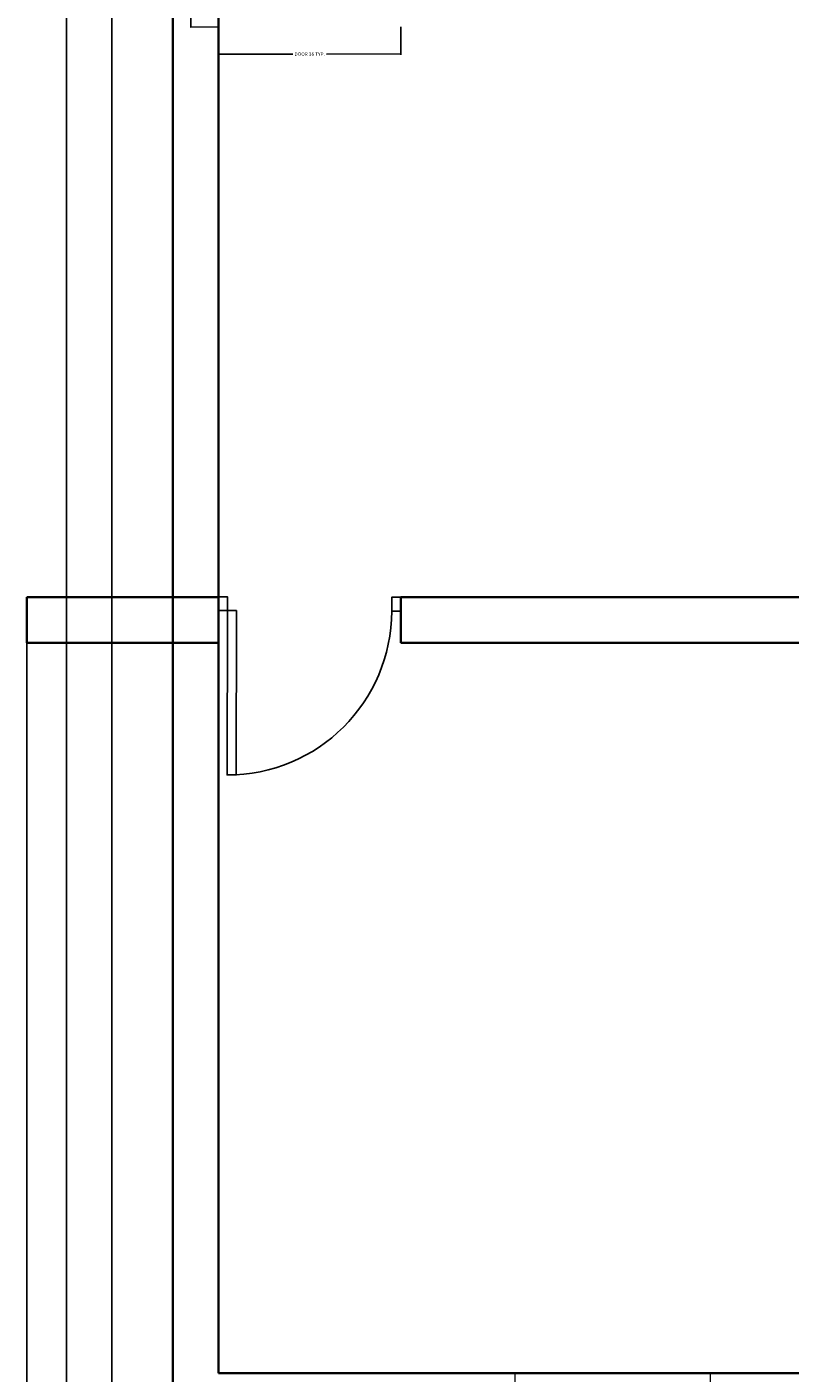
# Model space of a CAD drawing. Units: inches. Extents: x 867 to 1667, y -234 to 788.
# Tile 24 of 42: x 1366 to 1517, y -8 to 258. Entities that reach past the tile are written whole.
import ezdxf

# ---------------------------------------------------------------- set-up
doc = ezdxf.new("R2010")
doc.units = ezdxf.units.IN
doc.header["$MEASUREMENT"] = 0
for name, color, linetype, lineweight in [('A-ANNO-DIMS', 2, 'Continuous', 18), ('A-Door', 150, 'Continuous', 25), ('A-Glaz', 92, 'Continuous', 18), ('A-Wall', 7, 'Continuous', 35)]:
    doc.layers.add(name, color=color, linetype=linetype, lineweight=lineweight)
doc.layers.add('NET 01', color=8, linetype='Continuous')
doc.styles.get("Standard").update_dxf_attribs({"font": 'arial.ttf'})
doc.dimstyles.get("Standard").update_dxf_attribs({"dimtxt": 0.6875, "dimasz": 0.18, "dimexe": 0.18, "dimexo": 0.0625, "dimgap": 0.09, "dimtad": 0, "dimdec": 4, "dimzin": 0, "dimdsep": 46, "dimlunit": 4, "dimtxsty": 'Standard', "dimcen": 0.09, "dimadec": 0, "dimazin": 0, "dimtfac": 1, "dimtdec": 4, "dimtofl": 0, "dimtmove": 0, "dimatfit": 3, "dimfxl": 1, "dimtolj": 1, "dimtzin": 0, "dimarcsym": 0})

# ---------------------------------------------------------------- blocks, each defined once
blk = doc.blocks.new('A$C292B336C')
at = {"layer": 'A-Door'}
for points in [[(-0.05, 0), (-0.05, 0.9), (0, 0.9), (0, 0)], [(-0.95, 0), (-0.95, -0.075), (-0.9, -0.075), (-0.9, 0)], [(0, 0), (0, -0.075), (0.05, -0.075), (0.05, 0)]]:
    blk.add_lwpolyline(points, close=True, dxfattribs=at)
at = {"layer": 'NET 01'}
blk.add_arc((0, 0), 0.9, 90, 180, dxfattribs=at)
blk = doc.blocks.new('WIN-38_58IN')
for p, q in [((0, 9), (0, 0)), ((38.58, 0), (38.58, 9)), ((0, 6), (38.58, 6)), ((0, 2.92), (38.58, 2.92)), ((0, 0), (38.58, 0))]:
    blk.add_line(p, q)
blk = doc.blocks.new('*D5')
at = {"layer": 'A-ANNO-DIMS', "color": 0, "lineweight": -2, "transparency": 16777216}
for p, q in [((1403.89, 257.55), (1403.9, 252.04)), ((1439.9, 257.64), (1439.91, 252.12)), ((1404.08, 252.22), (1418.58, 252.25)), ((1439.73, 252.3), (1425.22, 252.26))]:
    blk.add_line(p, q, dxfattribs=at)
at = {"layer": 'A-ANNO-DIMS', "color": 0, "transparency": 16777216}
for points in [[(1404.08, 252.25), (1404.08, 252.19), (1403.9, 252.22)], [(1439.73, 252.33), (1439.73, 252.27), (1439.91, 252.3)]]:
    blk.add_solid(points, dxfattribs=at)
at = {"layer": 'Defpoints', "color": 0, "transparency": 16777216}
for p in [(1403.89, 257.62), (1439.9, 257.7), (1403.9, 252.22)]:
    blk.add_point(p, dxfattribs=at)
at = {"layer": 'A-ANNO-DIMS', "color": 0, "transparency": 16777216, "insert": (1421.9, 252.26), "char_height": 0.6875, "attachment_point": 5, "rotation": 0.1281}
blk.add_mtext('\\A1;DOOR 36 TYP.', dxfattribs=at)
blk = doc.blocks.new('*D6')
at = {"layer": 'A-ANNO-DIMS', "color": 0, "lineweight": -2, "transparency": 16777216}
for p, q in [((1403.75, 292.73), (1398.23, 292.72)), ((1398.41, 292.54), (1398.44, 276.92)), ((1398.48, 257.78), (1398.45, 273.4)), ((1403.82, 257.62), (1398.3, 257.6))]:
    blk.add_line(p, q, dxfattribs=at)
at = {"layer": 'A-ANNO-DIMS', "color": 0, "transparency": 16777216}
for points in [[(1398.44, 292.54), (1398.38, 292.54), (1398.41, 292.72)], [(1398.51, 257.78), (1398.45, 257.78), (1398.48, 257.6)]]:
    blk.add_solid(points, dxfattribs=at)
at = {"layer": 'Defpoints', "color": 0, "transparency": 16777216}
for p in [(1398.41, 292.72), (1403.81, 292.73), (1403.89, 257.62)]:
    blk.add_point(p, dxfattribs=at)
at = {"layer": 'A-ANNO-DIMS', "color": 0, "transparency": 16777216, "insert": (1398.45, 275.16), "char_height": 0.6875, "attachment_point": 5, "rotation": 270.1281}
blk.add_mtext('\\A1;35 TYP.', dxfattribs=at)
blk = doc.blocks.new('*D23')
at = {"layer": 'A-ANNO-DIMS', "color": 0, "lineweight": -2, "transparency": 16777216}
for p, q in [((1373.89, 623.55), (1373.89, -233.54)), ((1382.89, 623.55), (1382.89, -233.54)), ((1374.07, -233.36), (1378.07, -233.36)), ((1382.71, -233.36), (1378.7, -233.36))]:
    blk.add_line(p, q, dxfattribs=at)
at = {"layer": 'A-ANNO-DIMS', "color": 0, "transparency": 16777216}
for points in [[(1374.07, -233.33), (1374.07, -233.39), (1373.89, -233.36)], [(1382.71, -233.33), (1382.71, -233.39), (1382.89, -233.36)]]:
    blk.add_solid(points, dxfattribs=at)
at = {"layer": 'Defpoints', "color": 0, "transparency": 16777216}
for p in [(1373.89, 623.62), (1382.89, 623.62), (1382.89, -233.36)]:
    blk.add_point(p, dxfattribs=at)
at = {"layer": 'A-ANNO-DIMS', "color": 0, "transparency": 16777216, "insert": (1378.39, -233.36), "char_height": 0.688, "attachment_point": 5}
blk.add_mtext('\\A1;9', dxfattribs=at)
blk = doc.blocks.new('*D60')
at = {"layer": 'A-ANNO-DIMS', "color": 0, "lineweight": -2, "transparency": 16777216}
for p, q in [((1366.11, 136.05), (1366.11, -233.54)), ((1394.89, 136.05), (1394.89, -233.54)), ((1366.29, -233.36), (1379.24, -233.36)), ((1394.71, -233.36), (1381.75, -233.36))]:
    blk.add_line(p, q, dxfattribs=at)
at = {"layer": 'A-ANNO-DIMS', "color": 0, "transparency": 16777216}
for points in [[(1366.29, -233.33), (1366.29, -233.39), (1366.11, -233.36)], [(1394.71, -233.33), (1394.71, -233.39), (1394.89, -233.36)]]:
    blk.add_solid(points, dxfattribs=at)
at = {"layer": 'Defpoints', "color": 0, "transparency": 16777216}
for p in [(1366.11, 136.12), (1394.89, 136.12), (1394.89, -233.36)]:
    blk.add_point(p, dxfattribs=at)
at = {"layer": 'A-ANNO-DIMS', "color": 0, "transparency": 16777216, "insert": (1380.5, -233.36), "char_height": 0.688, "attachment_point": 5}
blk.add_mtext('\\A1;28.78', dxfattribs=at)

msp = doc.modelspace()

# ---------------------------------------------------------------- linework, layer by layer
at = {"layer": 'A-Wall'}
for p, q in [((1394.8866, 413.617), (1394.8866, 136.117)), ((1403.8866, 413.617), (1403.8866, 136.117)), ((1394.8866, 221.617), (1394.8866, -16.883)), ((1403.8866, 221.617), (1403.8866, -7.883)), ((1403.8866, 145.117), (1366.1114, 145.117)), ((1366.1114, 145.117), (1366.1114, 136.117)), ((1568.8866, 145.117), (1439.8866, 145.117)), ((1439.8866, 145.117), (1439.8866, 136.117)), ((1403.8866, 136.117), (1366.1114, 136.117)), ((1559.8866, 136.117), (1439.8866, 136.117)), ((1559.8866, -7.883), (1403.8866, -7.883))]:
    msp.add_line(p, q, dxfattribs=at)

# ---------------------------------------------------------------- block references
at = {"layer": 'A-Door', "xscale": 36.01171521992244, "yscale": 36.01171521992244, "zscale": 36.01171521992244, "rotation": 179.8718688753832}
msp.add_blockref('A$C292B336C', (1405.6812, 142.4927), dxfattribs=at)
at = {"layer": 'A-Glaz'}
msp.add_blockref('WIN-38_58IN', (1462.3871, -16.883), dxfattribs=at)

# ---------------------------------------------------------------- dimensions: what is measured, and where the dimension line sits
at = {"layer": 'A-ANNO-DIMS'}
for base, p1, p2, override, picture, middle in [((1382.8866, -233.3581), (1373.8866, 623.617), (1382.8866, 623.617), {"dimdec": 0, "dimlfac": 1, "dimrnd": 0, "dimzin": 0, "dimdsep": 46, "dimlunit": 2}, '*D23', (1378.3866, -233.3581)), ((1394.8866, -233.3581), (1366.1051, 136.117), (1394.8866, 136.117), {"dimdec": 2, "dimlfac": 1, "dimrnd": 0, "dimzin": 0, "dimdsep": 46, "dimlunit": 2}, '*D60', (1380.4959, -233.3581))]:
    dim = msp.add_linear_dim(base=base, p1=p1, p2=p2, dimstyle='Standard', override=override, dxfattribs=at)
    dim.commit()
    dim.dimension.update_dxf_attribs({"geometry": picture, "text_midpoint": middle})
for base, p1, p2, angle, text, picture, middle in [((1398.4064, 292.7163), (1403.8866, 257.617), (1403.8081, 292.7284), 90.128131, '<> TYP.', '*D6', (1398.4456, 275.1606)), ((1403.8987, 252.2153), (1439.8983, 257.6976), (1403.8866, 257.617), 180.128131, 'DOOR <> TYP.', '*D5', (1421.9045, 252.2556))]:
    dim = msp.add_linear_dim(base=base, p1=p1, p2=p2, angle=angle, text=text, dimstyle='Standard', override={"dimdec": 0, "dimlfac": 1, "dimrnd": 0, "dimzin": 0, "dimdsep": 46, "dimlunit": 2}, dxfattribs=at)
    dim.commit()
    dim.dimension.update_dxf_attribs({"geometry": picture, "text_midpoint": middle})

doc.saveas('drawing.dxf')
